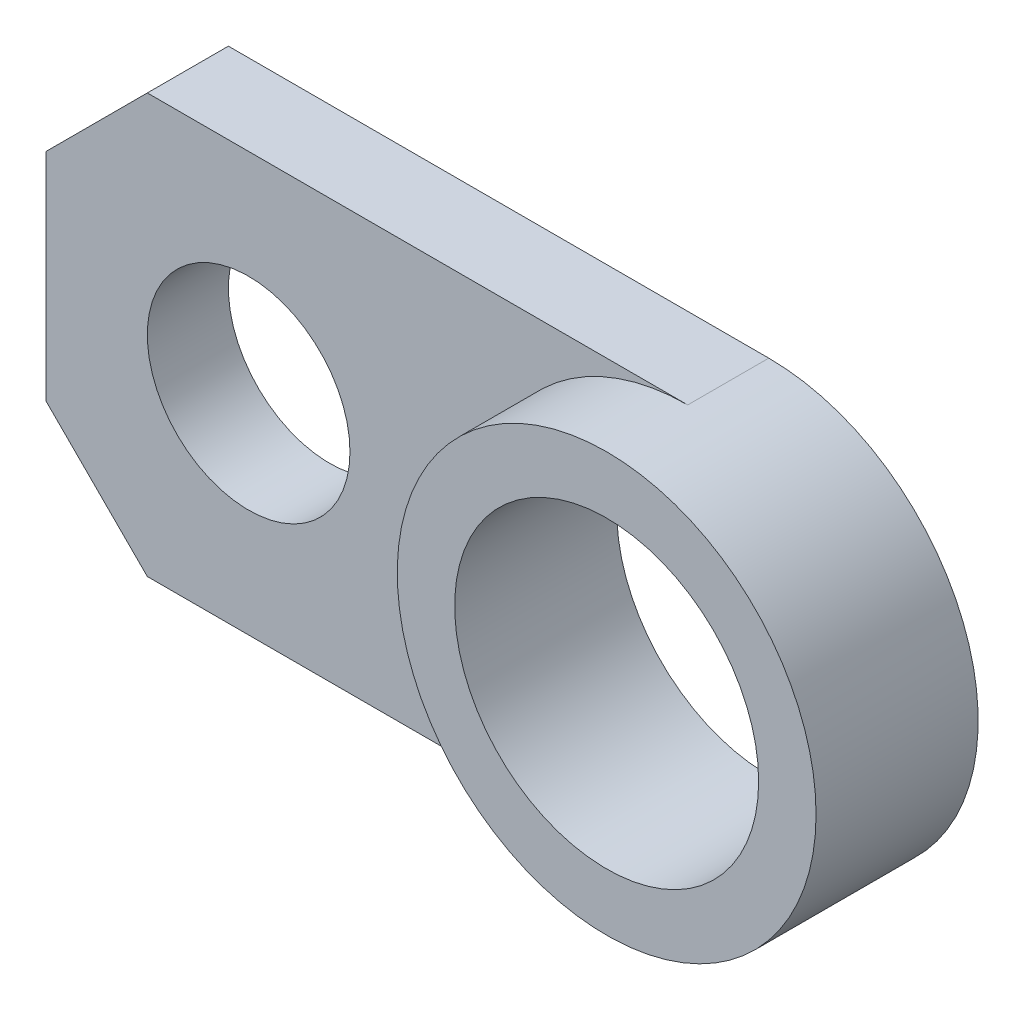
ISO-10303-21;
HEADER;
FILE_DESCRIPTION(('STEP AP214'),'2;1');
FILE_NAME('part.step','',(''),(''),'','','');
FILE_SCHEMA(('AUTOMOTIVE_DESIGN { 1 0 10303 214 1 1 1 1 }'));
ENDSEC;
DATA;
#1=APPLICATION_CONTEXT('core data for automotive mechanical design processes');
#2=APPLICATION_PROTOCOL_DEFINITION('international standard','automotive_design',2000,#1);
#3=PRODUCT_CONTEXT('',#1,'mechanical');
#4=PRODUCT('Part','Part','',(#3));
#5=PRODUCT_RELATED_PRODUCT_CATEGORY('part','',(#4));
#6=PRODUCT_DEFINITION_FORMATION('','',#4);
#7=PRODUCT_DEFINITION_CONTEXT('part definition',#1,'design');
#8=PRODUCT_DEFINITION('design','',#6,#7);
#9=PRODUCT_DEFINITION_SHAPE('','',#8);
#10=(LENGTH_UNIT() NAMED_UNIT(*) SI_UNIT(.MILLI.,.METRE.));
#11=(NAMED_UNIT(*) PLANE_ANGLE_UNIT() SI_UNIT($,.RADIAN.));
#12=(NAMED_UNIT(*) SI_UNIT($,.STERADIAN.) SOLID_ANGLE_UNIT());
#13=UNCERTAINTY_MEASURE_WITH_UNIT(LENGTH_MEASURE(1.E-05),#10,'distance_accuracy_value','');
#14=(GEOMETRIC_REPRESENTATION_CONTEXT(3) GLOBAL_UNCERTAINTY_ASSIGNED_CONTEXT((#13)) GLOBAL_UNIT_ASSIGNED_CONTEXT((#10,
#11,#12)) REPRESENTATION_CONTEXT('',''));
#15=CARTESIAN_POINT('',(0.,0.,0.));
#16=DIRECTION('',(0.,0.,1.));
#17=DIRECTION('',(1.,0.,0.));
#18=AXIS2_PLACEMENT_3D('',#15,#16,#17);
#19=CARTESIAN_POINT('',(0.,-31.,12.));
#20=DIRECTION('',(0.,-1.,0.));
#21=DIRECTION('',(0.,0.,-1.));
#22=AXIS2_PLACEMENT_3D('',#19,#20,#21);
#23=PLANE('',#22);
#24=DIRECTION('',(-1.,0.,0.));
#25=VECTOR('',#24,1.);
#26=CARTESIAN_POINT('',(0.,-31.,0.));
#27=LINE('',#26,#25);
#28=CARTESIAN_POINT('',(65.,-31.,0.));
#29=VERTEX_POINT('',#28);
#30=CARTESIAN_POINT('',(-15.,-31.,0.));
#31=VERTEX_POINT('',#30);
#32=EDGE_CURVE('E129',#29,#31,#27,.T.);
#33=ORIENTED_EDGE('',*,*,#32,.F.);
#34=DIRECTION('',(0.,0.,-1.));
#35=VECTOR('',#34,1.);
#36=CARTESIAN_POINT('',(65.,-31.,12.));
#37=LINE('',#36,#35);
#38=CARTESIAN_POINT('',(65.,-31.,12.));
#39=VERTEX_POINT('',#38);
#40=EDGE_CURVE('E11',#39,#29,#37,.T.);
#41=ORIENTED_EDGE('',*,*,#40,.F.);
#42=DIRECTION('',(-1.,0.,0.));
#43=VECTOR('',#42,1.);
#44=CARTESIAN_POINT('',(0.,-31.,12.));
#45=LINE('',#44,#43);
#46=CARTESIAN_POINT('',(-15.,-31.,12.));
#47=VERTEX_POINT('',#46);
#48=EDGE_CURVE('E142',#39,#47,#45,.T.);
#49=ORIENTED_EDGE('',*,*,#48,.T.);
#50=DIRECTION('',(0.,0.,-1.));
#51=VECTOR('',#50,1.);
#52=CARTESIAN_POINT('',(-15.,-31.,12.));
#53=LINE('',#52,#51);
#54=EDGE_CURVE('E64',#47,#31,#53,.T.);
#55=ORIENTED_EDGE('',*,*,#54,.T.);
#56=EDGE_LOOP('',(#33,#41,#49,#55));
#57=FACE_BOUND('',#56,.T.);
#58=ADVANCED_FACE('F50',(#57),#23,.T.);
#59=CARTESIAN_POINT('',(65.,0.,12.));
#60=DIRECTION('',(0.,0.,-1.));
#61=DIRECTION('',(-1.,0.,0.));
#62=AXIS2_PLACEMENT_3D('',#59,#60,#61);
#63=CYLINDRICAL_SURFACE('',#62,31.);
#64=CARTESIAN_POINT('',(65.,0.,0.));
#65=DIRECTION('',(0.,0.,1.));
#66=DIRECTION('',(1.,0.,0.));
#67=AXIS2_PLACEMENT_3D('',#64,#65,#66);
#68=CIRCLE('',#67,31.);
#69=CARTESIAN_POINT('',(65.,31.,0.));
#70=VERTEX_POINT('',#69);
#71=EDGE_CURVE('E133',#29,#70,#68,.T.);
#72=ORIENTED_EDGE('',*,*,#71,.T.);
#73=DIRECTION('',(0.,0.,-1.));
#74=VECTOR('',#73,1.);
#75=CARTESIAN_POINT('',(65.,31.,12.));
#76=LINE('',#75,#74);
#77=CARTESIAN_POINT('',(65.,31.,12.));
#78=VERTEX_POINT('',#77);
#79=EDGE_CURVE('E57',#78,#70,#76,.T.);
#80=ORIENTED_EDGE('',*,*,#79,.F.);
#81=CARTESIAN_POINT('',(65.,0.,12.));
#82=DIRECTION('',(0.,0.,1.));
#83=DIRECTION('',(1.,0.,0.));
#84=AXIS2_PLACEMENT_3D('',#81,#82,#83);
#85=CIRCLE('',#84,31.);
#86=EDGE_CURVE('E335',#78,#39,#85,.T.);
#87=ORIENTED_EDGE('',*,*,#86,.T.);
#88=ORIENTED_EDGE('',*,*,#40,.T.);
#89=EDGE_LOOP('',(#72,#80,#87,#88));
#90=FACE_BOUND('',#89,.T.);
#91=CARTESIAN_POINT('',(65.,0.,24.));
#92=DIRECTION('',(0.,0.,1.));
#93=DIRECTION('',(1.,0.,0.));
#94=AXIS2_PLACEMENT_3D('',#91,#92,#93);
#95=CIRCLE('',#94,31.);
#96=CARTESIAN_POINT('',(96.,0.,24.));
#97=VERTEX_POINT('',#96);
#98=EDGE_CURVE('E135',#97,#97,#95,.T.);
#99=ORIENTED_EDGE('',*,*,#98,.F.);
#100=EDGE_LOOP('',(#99));
#101=FACE_BOUND('',#100,.T.);
#102=ADVANCED_FACE('F166',(#90,#101),#63,.T.);
#103=CARTESIAN_POINT('',(0.,31.,12.));
#104=DIRECTION('',(0.,-1.,0.));
#105=DIRECTION('',(0.,0.,-1.));
#106=AXIS2_PLACEMENT_3D('',#103,#104,#105);
#107=PLANE('',#106);
#108=DIRECTION('',(-1.,0.,0.));
#109=VECTOR('',#108,1.);
#110=CARTESIAN_POINT('',(0.,31.,0.));
#111=LINE('',#110,#109);
#112=CARTESIAN_POINT('',(-15.,31.,0.));
#113=VERTEX_POINT('',#112);
#114=EDGE_CURVE('E134',#70,#113,#111,.T.);
#115=ORIENTED_EDGE('',*,*,#114,.T.);
#116=DIRECTION('',(0.,0.,-1.));
#117=VECTOR('',#116,1.);
#118=CARTESIAN_POINT('',(-15.,31.,12.));
#119=LINE('',#118,#117);
#120=CARTESIAN_POINT('',(-15.,31.,12.));
#121=VERTEX_POINT('',#120);
#122=EDGE_CURVE('E122',#121,#113,#119,.T.);
#123=ORIENTED_EDGE('',*,*,#122,.F.);
#124=DIRECTION('',(-1.,0.,0.));
#125=VECTOR('',#124,1.);
#126=CARTESIAN_POINT('',(0.,31.,12.));
#127=LINE('',#126,#125);
#128=EDGE_CURVE('E108',#78,#121,#127,.T.);
#129=ORIENTED_EDGE('',*,*,#128,.F.);
#130=ORIENTED_EDGE('',*,*,#79,.T.);
#131=EDGE_LOOP('',(#115,#123,#129,#130));
#132=FACE_BOUND('',#131,.T.);
#133=ADVANCED_FACE('F147',(#132),#107,.F.);
#134=CARTESIAN_POINT('',(-23.,23.,12.));
#135=DIRECTION('',(0.707106781186547,-0.707106781186548,0.));
#136=DIRECTION('',(0.707106781186548,0.707106781186547,0.));
#137=AXIS2_PLACEMENT_3D('',#134,#135,#136);
#138=PLANE('',#137);
#139=DIRECTION('',(-0.707106781186548,-0.707106781186547,0.));
#140=VECTOR('',#139,1.);
#141=CARTESIAN_POINT('',(-23.,23.,0.));
#142=LINE('',#141,#140);
#143=CARTESIAN_POINT('',(-30.,16.,0.));
#144=VERTEX_POINT('',#143);
#145=EDGE_CURVE('E116',#113,#144,#142,.T.);
#146=ORIENTED_EDGE('',*,*,#145,.T.);
#147=DIRECTION('',(0.,0.,-1.));
#148=VECTOR('',#147,1.);
#149=CARTESIAN_POINT('',(-30.,16.,12.));
#150=LINE('',#149,#148);
#151=CARTESIAN_POINT('',(-30.,16.,12.));
#152=VERTEX_POINT('',#151);
#153=EDGE_CURVE('E113',#152,#144,#150,.T.);
#154=ORIENTED_EDGE('',*,*,#153,.F.);
#155=DIRECTION('',(-0.707106781186548,-0.707106781186547,0.));
#156=VECTOR('',#155,1.);
#157=CARTESIAN_POINT('',(-23.,23.,12.));
#158=LINE('',#157,#156);
#159=EDGE_CURVE('E101',#121,#152,#158,.T.);
#160=ORIENTED_EDGE('',*,*,#159,.F.);
#161=ORIENTED_EDGE('',*,*,#122,.T.);
#162=EDGE_LOOP('',(#146,#154,#160,#161));
#163=FACE_BOUND('',#162,.T.);
#164=ADVANCED_FACE('F118',(#163),#138,.F.);
#165=CARTESIAN_POINT('',(-30.,0.,12.));
#166=DIRECTION('',(-1.,0.,0.));
#167=DIRECTION('',(0.,0.,1.));
#168=AXIS2_PLACEMENT_3D('',#165,#166,#167);
#169=PLANE('',#168);
#170=DIRECTION('',(0.,1.,0.));
#171=VECTOR('',#170,1.);
#172=CARTESIAN_POINT('',(-30.,0.,0.));
#173=LINE('',#172,#171);
#174=CARTESIAN_POINT('',(-30.,-16.,0.));
#175=VERTEX_POINT('',#174);
#176=EDGE_CURVE('E140',#175,#144,#173,.T.);
#177=ORIENTED_EDGE('',*,*,#176,.F.);
#178=DIRECTION('',(0.,0.,-1.));
#179=VECTOR('',#178,1.);
#180=CARTESIAN_POINT('',(-30.,-16.,12.));
#181=LINE('',#180,#179);
#182=CARTESIAN_POINT('',(-30.,-16.,12.));
#183=VERTEX_POINT('',#182);
#184=EDGE_CURVE('E84',#183,#175,#181,.T.);
#185=ORIENTED_EDGE('',*,*,#184,.F.);
#186=DIRECTION('',(0.,1.,0.));
#187=VECTOR('',#186,1.);
#188=CARTESIAN_POINT('',(-30.,0.,12.));
#189=LINE('',#188,#187);
#190=EDGE_CURVE('E110',#183,#152,#189,.T.);
#191=ORIENTED_EDGE('',*,*,#190,.T.);
#192=ORIENTED_EDGE('',*,*,#153,.T.);
#193=EDGE_LOOP('',(#177,#185,#191,#192));
#194=FACE_BOUND('',#193,.T.);
#195=ADVANCED_FACE('F123',(#194),#169,.T.);
#196=CARTESIAN_POINT('',(-23.,-23.,12.));
#197=DIRECTION('',(-0.707106781186547,-0.707106781186548,0.));
#198=DIRECTION('',(0.707106781186548,-0.707106781186547,0.));
#199=AXIS2_PLACEMENT_3D('',#196,#197,#198);
#200=PLANE('',#199);
#201=DIRECTION('',(-0.707106781186548,0.707106781186547,0.));
#202=VECTOR('',#201,1.);
#203=CARTESIAN_POINT('',(-23.,-23.,0.));
#204=LINE('',#203,#202);
#205=EDGE_CURVE('E139',#31,#175,#204,.T.);
#206=ORIENTED_EDGE('',*,*,#205,.F.);
#207=ORIENTED_EDGE('',*,*,#54,.F.);
#208=DIRECTION('',(-0.707106781186548,0.707106781186547,0.));
#209=VECTOR('',#208,1.);
#210=CARTESIAN_POINT('',(-23.,-23.,12.));
#211=LINE('',#210,#209);
#212=EDGE_CURVE('E124',#47,#183,#211,.T.);
#213=ORIENTED_EDGE('',*,*,#212,.T.);
#214=ORIENTED_EDGE('',*,*,#184,.T.);
#215=EDGE_LOOP('',(#206,#207,#213,#214));
#216=FACE_BOUND('',#215,.T.);
#217=ADVANCED_FACE('F156',(#216),#200,.T.);
#218=CARTESIAN_POINT('',(0.,0.,12.));
#219=DIRECTION('',(0.,0.,1.));
#220=DIRECTION('',(1.,0.,0.));
#221=AXIS2_PLACEMENT_3D('',#218,#219,#220);
#222=PLANE('',#221);
#223=CARTESIAN_POINT('',(0.,0.,12.));
#224=DIRECTION('',(0.,0.,1.));
#225=DIRECTION('',(1.,0.,0.));
#226=AXIS2_PLACEMENT_3D('',#223,#224,#225);
#227=CIRCLE('',#226,15.);
#228=CARTESIAN_POINT('',(15.,0.,12.));
#229=VERTEX_POINT('',#228);
#230=EDGE_CURVE('E344',#229,#229,#227,.T.);
#231=ORIENTED_EDGE('',*,*,#230,.F.);
#232=EDGE_LOOP('',(#231));
#233=FACE_BOUND('',#232,.T.);
#234=ORIENTED_EDGE('',*,*,#86,.F.);
#235=ORIENTED_EDGE('',*,*,#128,.T.);
#236=ORIENTED_EDGE('',*,*,#159,.T.);
#237=ORIENTED_EDGE('',*,*,#190,.F.);
#238=ORIENTED_EDGE('',*,*,#212,.F.);
#239=ORIENTED_EDGE('',*,*,#48,.F.);
#240=EDGE_LOOP('',(#234,#235,#236,#237,#238,#239));
#241=FACE_BOUND('',#240,.T.);
#242=ADVANCED_FACE('F102',(#233,#241),#222,.T.);
#243=CARTESIAN_POINT('',(0.,0.,0.));
#244=DIRECTION('',(0.,0.,1.));
#245=DIRECTION('',(1.,0.,0.));
#246=AXIS2_PLACEMENT_3D('',#243,#244,#245);
#247=PLANE('',#246);
#248=CARTESIAN_POINT('',(0.,0.,0.));
#249=DIRECTION('',(0.,0.,1.));
#250=DIRECTION('',(1.,0.,0.));
#251=AXIS2_PLACEMENT_3D('',#248,#249,#250);
#252=CIRCLE('',#251,15.);
#253=CARTESIAN_POINT('',(15.,0.,0.));
#254=VERTEX_POINT('',#253);
#255=EDGE_CURVE('E49',#254,#254,#252,.T.);
#256=ORIENTED_EDGE('',*,*,#255,.T.);
#257=EDGE_LOOP('',(#256));
#258=FACE_BOUND('',#257,.T.);
#259=CARTESIAN_POINT('',(65.,0.,0.));
#260=DIRECTION('',(0.,0.,1.));
#261=DIRECTION('',(1.,0.,0.));
#262=AXIS2_PLACEMENT_3D('',#259,#260,#261);
#263=CIRCLE('',#262,22.5);
#264=CARTESIAN_POINT('',(87.5,0.,0.));
#265=VERTEX_POINT('',#264);
#266=EDGE_CURVE('E329',#265,#265,#263,.T.);
#267=ORIENTED_EDGE('',*,*,#266,.T.);
#268=EDGE_LOOP('',(#267));
#269=FACE_BOUND('',#268,.T.);
#270=ORIENTED_EDGE('',*,*,#32,.T.);
#271=ORIENTED_EDGE('',*,*,#205,.T.);
#272=ORIENTED_EDGE('',*,*,#176,.T.);
#273=ORIENTED_EDGE('',*,*,#145,.F.);
#274=ORIENTED_EDGE('',*,*,#114,.F.);
#275=ORIENTED_EDGE('',*,*,#71,.F.);
#276=EDGE_LOOP('',(#270,#271,#272,#273,#274,#275));
#277=FACE_BOUND('',#276,.T.);
#278=ADVANCED_FACE('F154',(#258,#269,#277),#247,.F.);
#279=CARTESIAN_POINT('',(65.,0.,24.));
#280=DIRECTION('',(0.,0.,1.));
#281=DIRECTION('',(1.,0.,0.));
#282=AXIS2_PLACEMENT_3D('',#279,#280,#281);
#283=PLANE('',#282);
#284=CARTESIAN_POINT('',(65.,0.,24.));
#285=DIRECTION('',(0.,0.,1.));
#286=DIRECTION('',(1.,0.,0.));
#287=AXIS2_PLACEMENT_3D('',#284,#285,#286);
#288=CIRCLE('',#287,22.5);
#289=CARTESIAN_POINT('',(87.5,0.,24.));
#290=VERTEX_POINT('',#289);
#291=EDGE_CURVE('E334',#290,#290,#288,.T.);
#292=ORIENTED_EDGE('',*,*,#291,.F.);
#293=EDGE_LOOP('',(#292));
#294=FACE_BOUND('',#293,.T.);
#295=ORIENTED_EDGE('',*,*,#98,.T.);
#296=EDGE_LOOP('',(#295));
#297=FACE_BOUND('',#296,.T.);
#298=ADVANCED_FACE('F199',(#294,#297),#283,.T.);
#299=CARTESIAN_POINT('',(65.,0.,-1.));
#300=DIRECTION('',(0.,0.,1.));
#301=DIRECTION('',(1.,0.,0.));
#302=AXIS2_PLACEMENT_3D('',#299,#300,#301);
#303=CYLINDRICAL_SURFACE('',#302,22.5);
#304=ORIENTED_EDGE('',*,*,#291,.T.);
#305=EDGE_LOOP('',(#304));
#306=FACE_BOUND('',#305,.T.);
#307=ORIENTED_EDGE('',*,*,#266,.F.);
#308=EDGE_LOOP('',(#307));
#309=FACE_BOUND('',#308,.T.);
#310=ADVANCED_FACE('F204',(#306,#309),#303,.F.);
#311=CARTESIAN_POINT('',(0.,0.,-13.));
#312=DIRECTION('',(0.,0.,1.));
#313=DIRECTION('',(1.,0.,0.));
#314=AXIS2_PLACEMENT_3D('',#311,#312,#313);
#315=CYLINDRICAL_SURFACE('',#314,15.);
#316=ORIENTED_EDGE('',*,*,#230,.T.);
#317=EDGE_LOOP('',(#316));
#318=FACE_BOUND('',#317,.T.);
#319=ORIENTED_EDGE('',*,*,#255,.F.);
#320=EDGE_LOOP('',(#319));
#321=FACE_BOUND('',#320,.T.);
#322=ADVANCED_FACE('F214',(#318,#321),#315,.F.);
#323=CLOSED_SHELL('',(#58,#102,#133,#164,#195,#217,#242,#278,#298,#310,#322));
#324=MANIFOLD_SOLID_BREP('B2',#323);
#325=ADVANCED_BREP_SHAPE_REPRESENTATION('',(#18,#324),#14);
#326=SHAPE_DEFINITION_REPRESENTATION(#9,#325);
ENDSEC;
END-ISO-10303-21;
